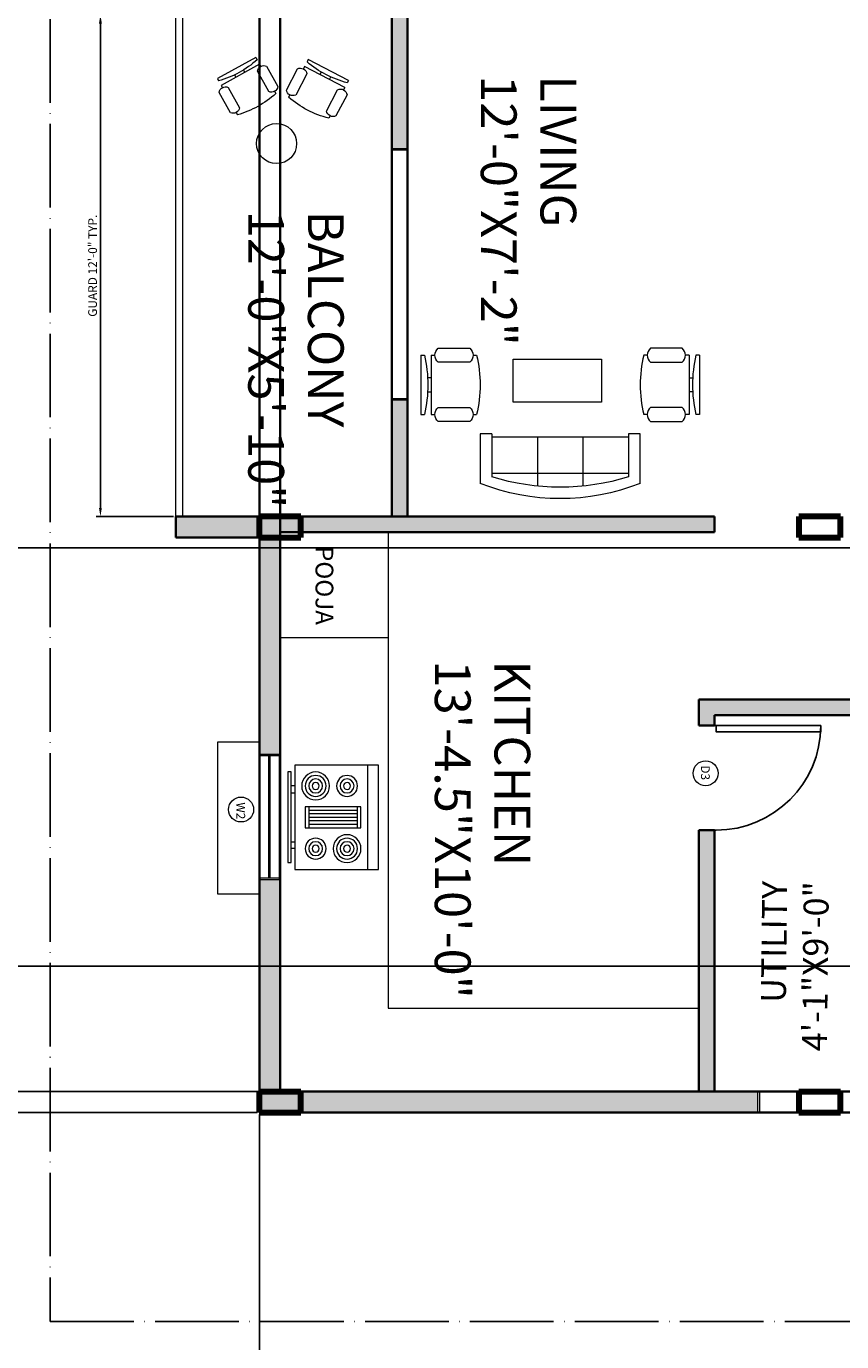
# Model space of a CAD drawing. Units: inches. Extents: x 7028582 to 7030319, y 63109697 to 63111305.
# Tile 4 of 18: x 7029168 to 7029402, y 63109901 to 63110278. Entities that reach past the tile are written whole.
import ezdxf

# ---------------------------------------------------------------- set-up
doc = ezdxf.new("R2010")
doc.units = ezdxf.units.IN
doc.linetypes.add('ACAD_ISO04W100', pattern=[30, 24, -3, 0, -3])
for name, color, linetype, lineweight in [('A-AREA-IDEN', 7, 'Continuous', 18), ('A-DOOR-IDEN', 20, 'Continuous', 13), ('A-EQPM', 9, 'Continuous', 18), ('A-FLOR-CASE', 9, 'Continuous', 18), ('A-FLOR-HRAL', 5, 'Continuous', 18), ('A-GLAZ-IDEN', 20, 'Continuous', 13), ('A-WALL-PATT', 8, 'Continuous', 13), ('C-ANNO-DIMS', 7, 'Continuous', 18), ('C-PROP', 1, 'ACAD_ISO04W100', 25), ('doors', 20, 'Continuous', 25), ('furniture', 9, 'Continuous', 18), ('PILLARS', 220, 'Continuous', 100), ('walls', 6, 'Continuous', 35), ('WINDOW SHADOW', 9, 'Continuous', 13), ('windows', 5, 'Continuous', 18)]:
    doc.layers.add(name, color=color, linetype=linetype, lineweight=lineweight)
doc.styles.get("Standard").update_dxf_attribs({"font": 'arial.ttf'})
doc.dimstyles.new('ISO-25', dxfattribs={"dimtxt": 2.5, "dimasz": 2.5, "dimexe": 1.25, "dimexo": 0.625, "dimtad": 1, "dimlunit": 4, "dimtxsty": 'Standard', "dimcen": 2.5, "dimadec": 0, "dimazin": 0, "dimtfac": 1, "dimtmove": 0, "dimatfit": 3, "dimfxl": 1, "dimarcsym": 0})

# ---------------------------------------------------------------- blocks, each defined once
blk = doc.blocks.new('*U2')
for p, q in [((0, 0), (0, -5)), ((30, 0), (30, -5))]:
    blk.add_line(p, q)
blk.add_lwpolyline([(0, 0), (0, 30), (1.75, 30), (1.75, 0)], close=True)
blk.add_arc((0, 0), 30, 0, 90)
blk = doc.blocks.new('Range-Oven - 30 in top')
for p, q in [((0, -3), (30, -3)), ((12, -6), (18, -6)), ((13, -20), (13, -6)), ((14, -6), (14, -20)), ((15, -20), (15, -6)), ((16, -6), (16, -20)), ((17, -20), (17, -6)), ((18, -20), (12, -20)), ((6, -24), (6, -25)), ((8, -25), (8, -24)), ((22, -25), (22, -24)), ((24, -24), (24, -25))]:
    blk.add_line(p, q)
for points in [[(0, -24), (0, 0), (30, 0), (30, -24)], [(12, -21), (12, -5), (18, -5), (18, -21)], [(2, -26), (2, -25), (28, -25), (28, -26)]]:
    blk.add_lwpolyline(points, close=True)
for centre, radius in [((6, -9), 4), ((6, -9), 3), ((6, -9), 2), ((24, -9), 3), ((24, -9), 2), ((6, -9), 1), ((24, -9), 1), ((6, -18), 3), ((24, -18), 4), ((24, -18), 3), ((6, -18), 2), ((6, -18), 1), ((24, -18), 2), ((24, -18), 1)]:
    blk.add_circle(centre, radius)
blk = doc.blocks.new('Chair - Desk')
for p, q in [((-8.5, 0), (-8.5, -1)), ((-8.5, 0), (8.5, 0)), ((8.5, 0), (8.5, -1)), ((-8.5, -3), (-8.5, -4)), ((-8.5, -3), (8.5, -3)), ((-2, -3), (-2, -1.9355)), ((2, -1.9576), (2, -3)), ((8.5, -3), (8.5, -4)), ((-10.5, -5), (-10.5, -14)), ((-6.5, -14), (-6.5, -5)), ((6.5, -5), (6.5, -14)), ((10.5, -14), (10.5, -5)), ((-8.5, -15), (-8.5, -16)), ((8.5, -15), (8.5, -16))]:
    blk.add_line(p, q)
for centre, radius, start, end in [((0, 34.625), 36.625, 256.5803, 283.4197), ((-8.5, -6.5), 2.5, 36.8699, 143.1301), ((8.5, -6.5), 2.5, 36.8699, 143.1301), ((-8.5, -12.5), 2.5, 216.8699, 323.1301), ((8.5, -12.5), 2.5, 216.8699, 323.1301), ((0, 19.625), 36.625, 256.5803, 283.4197)]:
    blk.add_arc(centre, radius, start, end)
blk = doc.blocks.new('Sofa - Roundback 7 ft.')
for p, q in [((-12.00002, -32.4421), (-12.00003, -6.5971)), ((11.99997, -32.4421), (11.99998, -6.5971)), ((-36.000027, -34), (-36.000027, -11.4696)), ((-35.999844, -13.3819), (35.9998, -13.3819)), ((35.99998, -34), (35.99998, -11.4696)), ((-36.000027, -32.4421), (35.99998, -32.4421))]:
    blk.add_line(p, q)
for points in [[(-36.000027, -34), (-42.000027, -34), (-42.000027, -8)], [(41.99998, -8), (41.99998, -34), (35.99998, -34)]]:
    blk.add_lwpolyline(points)
for centre, radius, start, end in [((0, -114.25), 114.25, 68.43141, 111.5686), ((-0.00001, -127.1968), 121.1968, 72.72033, 107.2797)]:
    blk.add_arc(centre, radius, start, end)
blk = doc.blocks.new('WIN-SASH-36')
for p, q in [((0, 36.05), (0, 0)), ((6, 35.55), (0, 35.55)), ((2.8, 35.55), (2.8, 0.5)), ((3.2, 35.55), (3.2, 0.5)), ((6, 0), (6, 36.05)), ((0, 0.5), (6, 0.5))]:
    blk.add_line(p, q)
blk = doc.blocks.new('WIN-SASH-24-FRAME')
for p, q in [((24.05, 6), (0, 6)), ((0.5, 6), (0.5, 0)), ((23.55, 0), (23.55, 6)), ((0, 0), (24.05, 0))]:
    blk.add_line(p, q)
blk = doc.blocks.new('WIN-SASH-BALCONY')
for p, q in [((0.13, 72.09), (0.13, 36.05)), ((4.63, 36.05), (4.63, 72.09)), ((4.63, 71.71), (0.13, 71.71)), ((0, 0.02), (0.13, 36.05)), ((0.13, 35.68), (0.13, 35.68)), ((4.63, 36.04), (4.5, 0)), ((4.5, 0.37), (0, 0.39))]:
    blk.add_line(p, q)
blk = doc.blocks.new('WINDOW-SHADE-SIDE-44')
for p, q in [((12, 43.55), (0, 43.55)), ((12, 0), (12, 43.55)), ((0, 0), (12, 0))]:
    blk.add_line(p, q)
blk = doc.blocks.new('KITCHEN-COUNTER')
for p, q in [((89.09, 136.54), (89.09, 16.65)), ((120, 106.35), (89.09, 106.35)), ((89.09, 16.65), (89.09, 0)), ((89.09, 0), (0, 0))]:
    blk.add_line(p, q)
blk = doc.blocks.new('COLUMN-RECT-PROFILE')
for p, q in [((11.91, 6), (0, 6)), ((0, 6), (0, 0)), ((11.91, 0), (11.91, 6)), ((0, 0), (11.91, 0))]:
    blk.add_line(p, q)
blk = doc.blocks.new('BALCONY-GUARD-12FT')
for p, q in [((0, 144), (0, 0)), ((2, 144), (2, 0))]:
    blk.add_line(p, q)
blk = doc.blocks.new('TABLE-COFFEE-RECT')
blk.add_lwpolyline([(25.34, 12.34), (0, 12.34), (0, 0), (25.34, 0)], close=True)
blk = doc.blocks.new('TAG-D3-ST-L')
blk.add_circle((3.58, 3.58), 3.58)
blk.add_text('D3', height=2.5, rotation=270).set_placement((2.27, 5.87))
blk = doc.blocks.new('TAG-W2-ST-L')
blk.add_circle((3.58, 3.58), 3.58)
blk.add_text('W2', height=2.5, rotation=270).set_placement((2.23, 5.64))
blk = doc.blocks.new('TABLE-BALCONY-ROUND')
blk.add_circle((5.75, 5.75), 5.75)
blk = doc.blocks.new('*D87')
at = {"layer": 'C-ANNO-DIMS', "color": 0, "lineweight": -2, "transparency": 16777216}
for p, q in [((7029210.08, 63110281.56), (7029187.86, 63110281.56)), ((7029189.11, 63110279.06), (7029189.11, 63110140.06)), ((7029210.08, 63110137.56), (7029187.86, 63110137.56))]:
    blk.add_line(p, q, dxfattribs=at)
at = {"layer": 'C-ANNO-DIMS', "color": 0, "lineweight": 100, "transparency": 16777216}
for points in [[(7029188.69, 63110279.06), (7029189.52, 63110279.06), (7029189.11, 63110281.56)], [(7029188.69, 63110140.06), (7029189.52, 63110140.06), (7029189.11, 63110137.56)]]:
    blk.add_solid(points, dxfattribs=at)
at = {"layer": 'Defpoints', "color": 0, "lineweight": 100, "transparency": 16777216}
for p in [(7029210.71, 63110281.56), (7029189.11, 63110137.56), (7029210.71, 63110137.56)]:
    blk.add_point(p, dxfattribs=at)
at = {"layer": 'C-ANNO-DIMS', "color": 0, "transparency": 16777216, "insert": (7029187.19, 63110209.56), "char_height": 2.5, "attachment_point": 5, "rotation": 90}
blk.add_mtext('GUARD 12\'-0" TYP.', dxfattribs=at)
blk = doc.blocks.new('*D99')
at = {"layer": 'C-ANNO-DIMS', "color": 0, "lineweight": -2, "transparency": 16777216}
for p, q in [((7029234.71, 63109965.93), (7029234.71, 63109697.14)), ((7030175.71, 63109965.93), (7030175.71, 63109697.14)), ((7029237.21, 63109698.39), (7030173.21, 63109698.39))]:
    blk.add_line(p, q, dxfattribs=at)
at = {"layer": 'C-ANNO-DIMS', "color": 0, "lineweight": 100, "transparency": 16777216}
for points in [[(7029237.21, 63109698.8), (7029237.21, 63109697.97), (7029234.71, 63109698.39)], [(7030173.21, 63109698.8), (7030173.21, 63109697.97), (7030175.71, 63109698.39)]]:
    blk.add_solid(points, dxfattribs=at)
at = {"layer": 'Defpoints', "color": 0, "lineweight": 100, "transparency": 16777216}
for p in [(7029234.71, 63109966.56), (7030175.71, 63109966.56), (7030175.71, 63109698.39)]:
    blk.add_point(p, dxfattribs=at)
at = {"layer": 'C-ANNO-DIMS', "color": 0, "transparency": 16777216, "insert": (7029705.21, 63109700.29), "char_height": 2.5, "attachment_point": 5}
blk.add_mtext('78\'-5"', dxfattribs=at)
blk = doc.blocks.new('*D100')
at = {"layer": 'C-ANNO-DIMS', "color": 0, "lineweight": -2, "transparency": 16777216}
for p, q in [((7029234.08, 63111033.06), (7028586.23, 63111033.06)), ((7028587.48, 63109969.06), (7028587.48, 63111030.56)), ((7029234.08, 63109966.56), (7028586.23, 63109966.56))]:
    blk.add_line(p, q, dxfattribs=at)
at = {"layer": 'C-ANNO-DIMS', "color": 0, "lineweight": 100, "transparency": 16777216}
for points in [[(7028587.06, 63111030.56), (7028587.89, 63111030.56), (7028587.48, 63111033.06)], [(7028587.06, 63109969.06), (7028587.89, 63109969.06), (7028587.48, 63109966.56)]]:
    blk.add_solid(points, dxfattribs=at)
at = {"layer": 'Defpoints', "color": 0, "lineweight": 100, "transparency": 16777216}
for p in [(7028587.48, 63111033.06), (7029234.71, 63111033.06), (7029234.71, 63109966.56)]:
    blk.add_point(p, dxfattribs=at)
at = {"layer": 'C-ANNO-DIMS', "color": 0, "transparency": 16777216, "insert": (7028585.56, 63110499.81), "char_height": 2.5, "attachment_point": 5, "rotation": 90}
blk.add_mtext('88\'-10 1/2"', dxfattribs=at)
blk = doc.blocks.new('*D109')
at = {"layer": 'C-ANNO-DIMS', "color": 0, "lineweight": -2, "transparency": 16777216}
for p, q in [((7029710.58, 63110128.56), (7028586.23, 63110128.56)), ((7028587.48, 63110126.06), (7028587.48, 63110011.06)), ((7029710.58, 63110008.56), (7028586.23, 63110008.56))]:
    blk.add_line(p, q, dxfattribs=at)
at = {"layer": 'C-ANNO-DIMS', "color": 0, "lineweight": 100, "transparency": 16777216}
for points in [[(7028587.06, 63110126.06), (7028587.89, 63110126.06), (7028587.48, 63110128.56)], [(7028587.06, 63110011.06), (7028587.89, 63110011.06), (7028587.48, 63110008.56)]]:
    blk.add_solid(points, dxfattribs=at)
at = {"layer": 'Defpoints', "color": 0, "lineweight": 100, "transparency": 16777216}
for p in [(7029711.21, 63110128.56), (7028587.48, 63110008.56), (7029711.21, 63110008.56)]:
    blk.add_point(p, dxfattribs=at)
at = {"layer": 'C-ANNO-DIMS', "color": 0, "transparency": 16777216, "insert": (7028585.57, 63110068.56), "char_height": 2.5, "attachment_point": 5, "rotation": 90}
blk.add_mtext('10\'-0"', dxfattribs=at)
blk = doc.blocks.new('*D110')
at = {"layer": 'C-ANNO-DIMS', "color": 0, "lineweight": -2, "transparency": 16777216}
for p, q in [((7029747.58, 63110008.56), (7028586.23, 63110008.56)), ((7028587.48, 63110006.06), (7028587.48, 63109975.06)), ((7029747.58, 63109972.56), (7028586.23, 63109972.56))]:
    blk.add_line(p, q, dxfattribs=at)
at = {"layer": 'C-ANNO-DIMS', "color": 0, "lineweight": 100, "transparency": 16777216}
for points in [[(7028587.06, 63110006.06), (7028587.89, 63110006.06), (7028587.48, 63110008.56)], [(7028587.06, 63109975.06), (7028587.89, 63109975.06), (7028587.48, 63109972.56)]]:
    blk.add_solid(points, dxfattribs=at)
at = {"layer": 'Defpoints', "color": 0, "lineweight": 100, "transparency": 16777216}
for p in [(7029748.21, 63110008.56), (7028587.48, 63109972.56), (7029748.21, 63109972.56)]:
    blk.add_point(p, dxfattribs=at)
at = {"layer": 'C-ANNO-DIMS', "color": 0, "transparency": 16777216, "insert": (7028585.57, 63109990.56), "char_height": 2.5, "attachment_point": 5, "rotation": 90}
blk.add_mtext('3\'-0"', dxfattribs=at)

msp = doc.modelspace()

# ---------------------------------------------------------------- hatches: boundary and pattern name
at = {"layer": 'A-WALL-PATT'}
h = msp.add_hatch(color=256, dxfattribs=at)
h.dxf.hatch_style = 1
h.paths.add_polyline_path([(7029272.705, 63110281.557), (7029277.205, 63110281.557), (7029277.205, 63110243.163), (7029272.705, 63110243.163)])
h = msp.add_hatch(color=256, dxfattribs=at)
h.dxf.hatch_style = 1
h.paths.add_polyline_path([(7029272.705, 63110137.557), (7029277.205, 63110137.557), (7029277.205, 63110171.09), (7029272.705, 63110171.074)])
h = msp.add_hatch(color=256, dxfattribs=at)
h.dxf.hatch_style = 1
h.paths.add_polyline_path([(7029210.705, 63110137.557), (7029210.705, 63110131.557), (7029234.705, 63110131.557), (7029234.705, 63110137.557)])
h = msp.add_hatch(color=256, dxfattribs=at)
h.dxf.hatch_style = 1
h.paths.add_polyline_path([(7029234.705, 63110137.557), (7029240.705, 63110137.557), (7029240.705, 63110069.386), (7029234.705, 63110069.386)])
h = msp.add_hatch(color=256, dxfattribs=at)
h.dxf.hatch_style = 1
h.paths.add_polyline_path([(7029240.705, 63110137.557), (7029240.705, 63110133.057), (7029365.205, 63110133.057), (7029365.205, 63110137.557)])
h = msp.add_hatch(color=256, dxfattribs=at)
h.dxf.hatch_style = 1
h.paths.add_polyline_path([(7029414.205, 63110080.557), (7029414.205, 63110085.057), (7029360.705, 63110085.057), (7029360.705, 63110077.557), (7029365.205, 63110077.557), (7029365.205, 63110080.557)])
h = msp.add_hatch(color=256, dxfattribs=at)
h.dxf.hatch_style = 1
h.paths.add_polyline_path([(7029234.705, 63109966.557), (7029377.666, 63109966.557), (7029377.666, 63109972.557), (7029365.205, 63109972.557), (7029365.205, 63110047.557), (7029360.705, 63110047.557), (7029360.705, 63109972.557), (7029240.705, 63109972.557), (7029240.705, 63110033.338), (7029234.705, 63110033.338)])

# ---------------------------------------------------------------- linework, layer by layer
at = {"layer": 'C-PROP'}
for p, q in [((7029174.705, 63111093.057), (7029174.705, 63109906.557)), ((7029174.705, 63109906.557), (7030235.705, 63109906.557))]:
    msp.add_line(p, q, dxfattribs=at)
at = {"layer": 'walls'}
for p, q in [((7029234.705, 63110716.557), (7029234.705, 63109966.557)), ((7029240.705, 63110716.557), (7029240.705, 63109972.557)), ((7029272.705, 63110281.557), (7029272.705, 63110137.557)), ((7029277.205, 63110281.557), (7029277.205, 63110137.557)), ((7029210.705, 63110131.557), (7029210.705, 63110137.557)), ((7029210.705, 63110137.557), (7029234.705, 63110137.557)), ((7029234.705, 63109966.557), (7029234.705, 63110137.557)), ((7029234.705, 63109966.557), (7029234.705, 63110137.557)), ((7029234.705, 63110137.557), (7029365.205, 63110137.557)), ((7029240.705, 63109972.557), (7029240.705, 63110137.557)), ((7029240.705, 63109972.557), (7029240.705, 63110137.557)), ((7029365.205, 63110133.057), (7029365.205, 63110137.557)), ((7029234.705, 63110131.557), (7029210.705, 63110131.557)), ((7029240.705, 63110133.057), (7029365.205, 63110133.057)), ((7029360.705, 63110077.557), (7029360.705, 63110085.057)), ((7029360.705, 63110085.057), (7029445.705, 63110085.057)), ((7029365.205, 63110077.557), (7029365.205, 63110080.557)), ((7029365.205, 63110080.557), (7029445.705, 63110080.557)), ((7029365.205, 63110080.557), (7029365.205, 63110077.557)), ((7029365.205, 63110077.557), (7029360.705, 63110077.557)), ((7029360.705, 63109972.557), (7029360.705, 63110047.557)), ((7029360.705, 63110047.557), (7029365.205, 63110047.557)), ((7029365.205, 63109972.557), (7029365.205, 63110047.557)), ((7029240.705, 63109972.557), (7030169.705, 63109972.557)), ((7030169.705, 63109972.557), (7029240.705, 63109972.557)), ((7029240.705, 63109972.557), (7029360.705, 63109972.557)), ((7029365.205, 63109972.557), (7029414.205, 63109972.557)), ((7029234.705, 63109966.557), (7030175.705, 63109966.557)), ((7030175.705, 63109966.557), (7029234.705, 63109966.557)), ((7029234.705, 63109966.557), (7029662.205, 63109966.557))]:
    msp.add_line(p, q, dxfattribs=at)
at = {"layer": 'windows'}
for p, q in [((7029272.705, 63110243.163), (7029277.205, 63110243.163)), ((7029272.834, 63110171.074), (7029277.334, 63110171.09)), ((7029234.512, 63110069.386), (7029240.512, 63110069.386)), ((7029240.512, 63110033.338), (7029234.512, 63110033.338)), ((7029377.666, 63109966.557), (7029377.666, 63109972.557))]:
    msp.add_line(p, q, dxfattribs=at)

# ---------------------------------------------------------------- block references
at = {"layer": 'A-DOOR-IDEN'}
msp.add_blockref('TAG-D3-ST-L', (7029359.103, 63110060.309), dxfattribs=at)
at = {"layer": 'A-EQPM', "xscale": -1, "rotation": 270}
msp.add_blockref('Range-Oven - 30 in top', (7029268.844, 63110036.257), dxfattribs=at)
at = {"layer": 'A-FLOR-CASE', "extrusion": (0, 0, -1), "zscale": -1}
msp.add_blockref('KITCHEN-COUNTER', (-7029360.705, 63109996.518), dxfattribs=at)
at = {"layer": 'A-FLOR-HRAL', "rotation": 180}
msp.add_blockref('BALCONY-GUARD-12FT', (7029212.705, 63110281.557), dxfattribs=at)
at = {"layer": 'A-GLAZ-IDEN'}
msp.add_blockref('TAG-W2-ST-L', (7029225.884, 63110049.907), dxfattribs=at)
at = {"layer": 'doors', "rotation": 270}
msp.add_blockref('*U2', (7029365.705, 63110077.557), dxfattribs=at)
at = {"layer": 'furniture'}
for name, p, xscale, yscale, zscale, rotation in [('Chair - Desk', (7029228.177, 63110266.309), -0.740937522274531, 0.740937522274531, 0.740937522274531, 28.89971253738977), ('Chair - Desk', (7029254.497, 63110265.758), -0.7643373636972337, 0.7643373636972337, 0.7643373636972337, 332.4708086599736), ('Sofa - Roundback 7 ft.', (7029320.972, 63110142.72), -0.5455524879488546, 0.5455524879488546, 0.5455524879488546, 180)]:
    msp.add_blockref(name, p, dxfattribs=dict(at, xscale=xscale, yscale=yscale, zscale=zscale, rotation=rotation))
msp.add_blockref('TABLE-BALCONY-ROUND', (7029233.889, 63110238.874), dxfattribs=at)
at = {"layer": 'furniture', "xscale": -1, "rotation": 90}
msp.add_blockref('Chair - Desk', (7029281.016, 63110175.367), dxfattribs=at)
at = {"layer": 'furniture', "rotation": 270}
msp.add_blockref('Chair - Desk', (7029360.929, 63110175.367), dxfattribs=at)
at = {"layer": 'furniture', "extrusion": (0, 0, -1), "zscale": -1}
msp.add_blockref('TABLE-COFFEE-RECT', (-7029332.859, 63110170.363), dxfattribs=at)
at = {"layer": 'PILLARS'}
for p in [(7029234.659, 63110131.557), (7029389.44, 63110131.557), (7029234.659, 63109966.505), (7029389.44, 63109966.505)]:
    msp.add_blockref('COLUMN-RECT-PROFILE', p, dxfattribs=at)
at = {"layer": 'WINDOW SHADOW', "rotation": 180}
msp.add_blockref('WINDOW-SHADE-SIDE-44', (7029234.706, 63110072.829), dxfattribs=at)
at = {"layer": 'windows', "extrusion": (0, 0, -1), "zscale": -1}
msp.add_blockref('WIN-SASH-BALCONY', (-7029277.334, 63110171.074), dxfattribs=at)
at = {"layer": 'windows'}
for name, p in [('WIN-SASH-36', (7029234.512, 63110033.338)), ('WIN-SASH-24-FRAME', (7029377.666, 63109966.557))]:
    msp.add_blockref(name, p, dxfattribs=at)

# ---------------------------------------------------------------- texts
at = {"layer": 'A-AREA-IDEN'}
for s, width, gutter_width, insert, char_height, attachment_point, rotation in [('LIVING\\P12\'-0"X7\'-2"', 82.04322, 51.315, (7029298.218, 63110264.231), 10.26307, 7, 270), ('BALCONY\\P12\'-0"X5\'-10"', 82.04322, 51.315, (7029231.516, 63110225.354), 10.26307, 7, 270), ('POOJA', 15.69653, 25.463, (7029250.809, 63110129.117), 5.0926, 7, 270), ('KITCHEN\\P13\'-4.5"X10\'-0"', 82.04322, 51.315, (7029285.025, 63110096.255), 10.26307, 7, 270), ('UTILITY\\P4\'-1"X9\'-0"', 42.97461, 35.821, (7029378.929, 63110033.048), 7.16426, 3, 89.3536)]:
    msp.add_mtext_dynamic_manual_height_columns(s, width=width, gutter_width=gutter_width, heights=[0], dxfattribs=dict(at, insert=insert, char_height=char_height, attachment_point=attachment_point, rotation=rotation))

# ---------------------------------------------------------------- dimensions: what is measured, and where the dimension line sits
at = {"layer": 'C-ANNO-DIMS'}
for base, p1, p2, picture, middle in [((7028587.475, 63111033.057), (7029234.705, 63109966.557), (7029234.705, 63111033.057), '*D100', (7028585.558, 63110499.807)), ((7028587.475, 63110008.557), (7029711.205, 63110128.557), (7029711.205, 63110008.557), '*D109', (7028585.574, 63110068.557)), ((7028587.475, 63109972.557), (7029748.205, 63110008.557), (7029748.205, 63109972.557), '*D110', (7028585.573, 63109990.557))]:
    dim = msp.add_linear_dim(base=base, p1=p1, p2=p2, angle=90, dimstyle='ISO-25', override={"dimdec": 1, "dimlfac": 1, "dimrnd": 0, "dimzin": 1, "dimdsep": 46, "dimlunit": 4, "dimfrac": 2}, dxfattribs=at)
    dim.commit()
    dim.dimension.update_dxf_attribs({"geometry": picture, "text_midpoint": middle})
dim = msp.add_linear_dim(base=(7029189.105, 63110137.557), p1=(7029210.705, 63110281.557), p2=(7029210.705, 63110137.557), angle=270, text='GUARD <> TYP.', dimstyle='ISO-25', override={"dimdec": 1, "dimlfac": 1, "dimrnd": 0, "dimzin": 1, "dimdsep": 46, "dimlunit": 4, "dimfrac": 2}, dxfattribs=at)
dim.commit()
dim.dimension.update_dxf_attribs({"geometry": '*D87', "text_midpoint": (7029187.188, 63110209.557)})
dim = msp.add_linear_dim(base=(7030175.705, 63109698.385), p1=(7029234.705, 63109966.557), p2=(7030175.705, 63109966.557), dimstyle='ISO-25', override={"dimdec": 1, "dimlfac": 1, "dimrnd": 0, "dimzin": 1, "dimdsep": 46, "dimlunit": 4, "dimfrac": 2}, dxfattribs=at)
dim.commit()
dim.dimension.update_dxf_attribs({"geometry": '*D99', "text_midpoint": (7029705.205, 63109700.287)})

doc.saveas('drawing.dxf')
